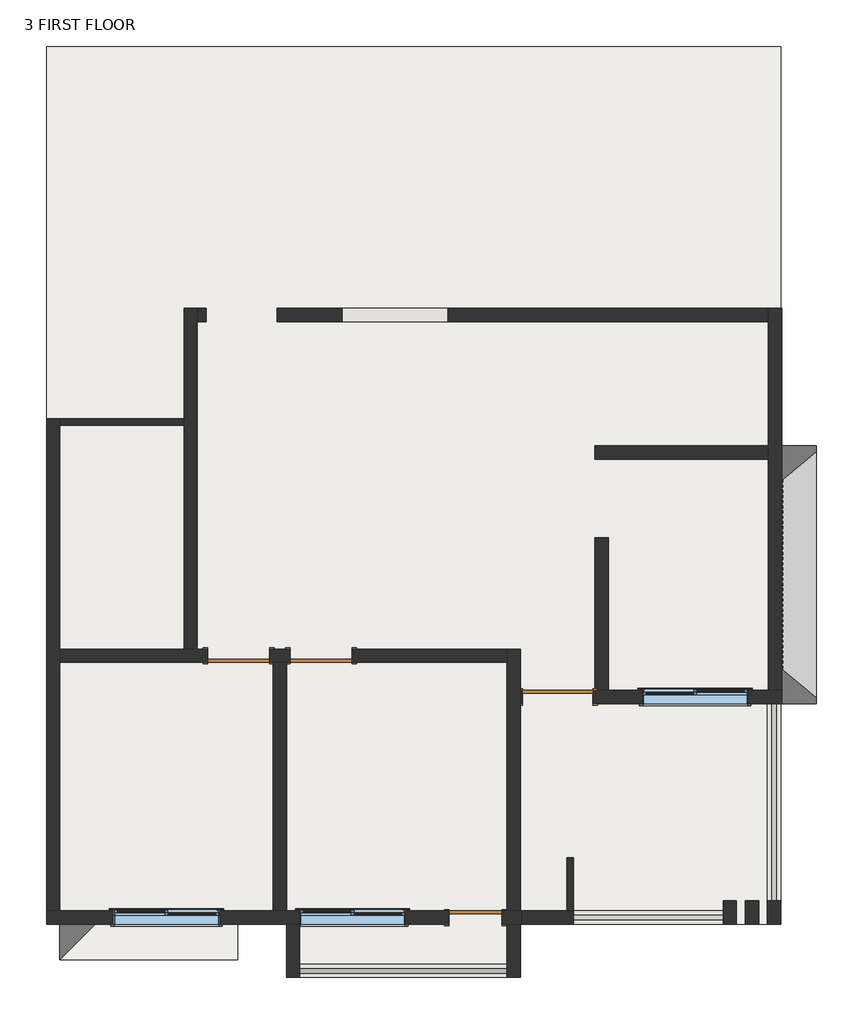
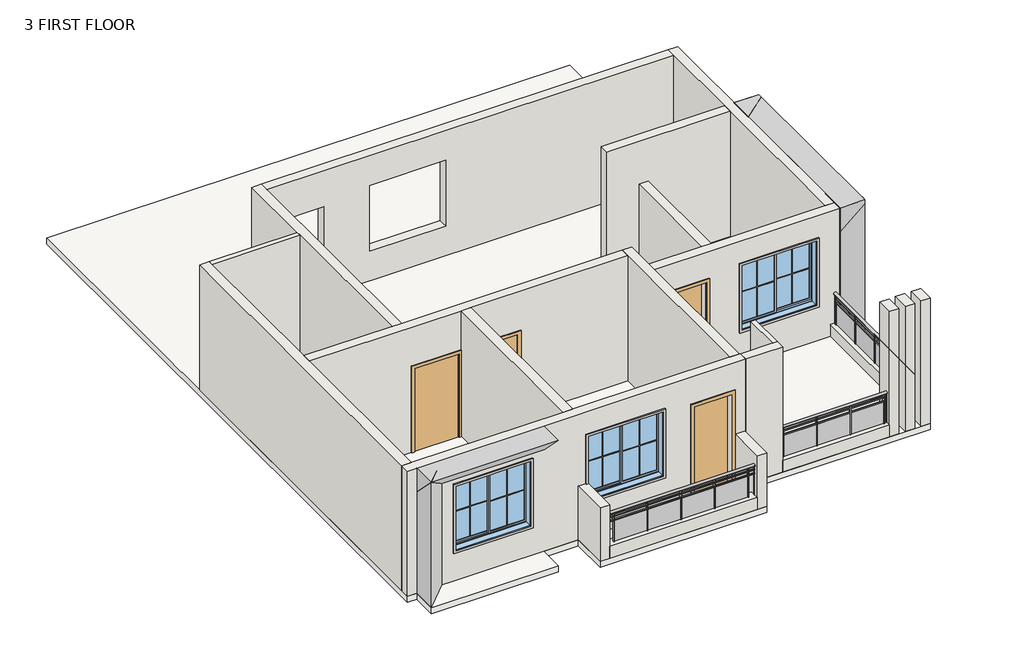
# One storey: 22 walls, 14 proxies, 4 doors, 3 railings, 3 windows, 1 slab.
# Revit data of these elements (continued)
# Elements 27, 28, 29, 30, 31, 32, 33, 34, 35, 44 (IfcWall, "9\"") (continued)
#   Base Constraint = 3 FIRST FLOOR
#   Top Constraint = 4 SECOND FLOOR BASE
#   Materials on its faces: "Default Wall"
# Elements 36, 37 (IfcWall, "9\"")
#   Top Offset = 0' - 0"
#   Base Offset = 0' - 0"
#   Unconnected Height = 4' - 6"
#   wall height = 4' - 6"
#   Phase Created = New Construction
#   Base Constraint = 3 FIRST FLOOR
#   Materials on its faces: "Default Wall"
# Elements 38, 42, 43 (IfcWall, "9\"")
#   Top Offset = 0' - 0"
#   Base Offset = 0' - 0"
#   Unconnected Height = 1' - 0"
#   wall height = 1' - 0"
#   Phase Created = New Construction
#   Base Constraint = 3 FIRST FLOOR
#   Materials on its faces: "Default Wall"
# Elements 39, 40, 41 (IfcWall, "9\"")
#   Top Offset = 0' - 0"
#   Base Offset = 0' - 0"
#   Unconnected Height = 10' - 6"
#   wall height = 10' - 6"
#   Phase Created = New Construction
#   Base Constraint = 3 FIRST FLOOR
#   Materials on its faces: "Default Wall"
# Element 45 (IfcWindow, "Window-Sliding-Double")
#   Mark = "5"
#   Window Inset = 0' - 0"
#   Interior Wall Closure = 0' - 2 3/4"
#   Frame Extension = 0' - 0 1/4"
#   Exterior Wall Closure = 0' - 1 1/4"
#   Interior Trim Visibility = yes
#   Indicator Visibility = yes
#   Exterior Trim Visibility = yes
#   Phase Created = New Construction
#   Materials on its faces: "Wood - Stained", "Glass", "Clad - White"
# Element 46 (IfcWindow, "Window-Sliding-Double")
#   Mark = "6"
#   Window Inset = 0' - 0"
#   Interior Wall Closure = 0' - 2 3/4"
#   Frame Extension = 0' - 0 1/4"
#   Exterior Wall Closure = 0' - 1 1/4"
#   Interior Trim Visibility = yes
#   Indicator Visibility = yes
#   Exterior Trim Visibility = yes
#   Phase Created = New Construction
#   Materials on its faces: "Wood - Stained", "Glass", "Clad - White"
# Element 47 (IfcWindow, "Window-Sliding-Double")
#   Mark = "7"
#   Window Inset = 0' - 0"
#   Interior Wall Closure = 0' - 2 3/4"
#   Frame Extension = 0' - 0 1/4"
#   Exterior Wall Closure = 0' - 1 1/4"
#   Interior Trim Visibility = yes
#   Indicator Visibility = yes
#   Exterior Trim Visibility = yes
#   Phase Created = New Construction
#   Materials on its faces: "Wood - Stained", "Glass", "Clad - White"
# Materials
#   "Door - Panel": class "Wood", colour RGB 210 159 95, transparency 0, Cost = 0
#   "Door - Frame": colour RGB 118 70 51, transparency 0, Cost = 0
#   "Wood - Stained": class "Wood", colour RGB 224 178 126, transparency 0, Cost = 0
#   "Glass": class "Glass", colour RGB 0 128 192, transparency 0.75, Description = "Soda Lime Glass", Cost = 0
#   "Clad - White": class "Wood", colour RGB 242 242 238, transparency 0, Cost = 0
#   "Default New Material": class "Generic", colour RGB 64 128 128, transparency 0, Cost = 0
#   "Default Floor": colour RGB 128 128 128, transparency 0, Cost = 0
#   "Default Wall": colour RGB 128 128 128, transparency 0, Cost = 0
#   "outer wall": class "Generic", colour RGB 85 88 91, transparency 0, Cost = 0
